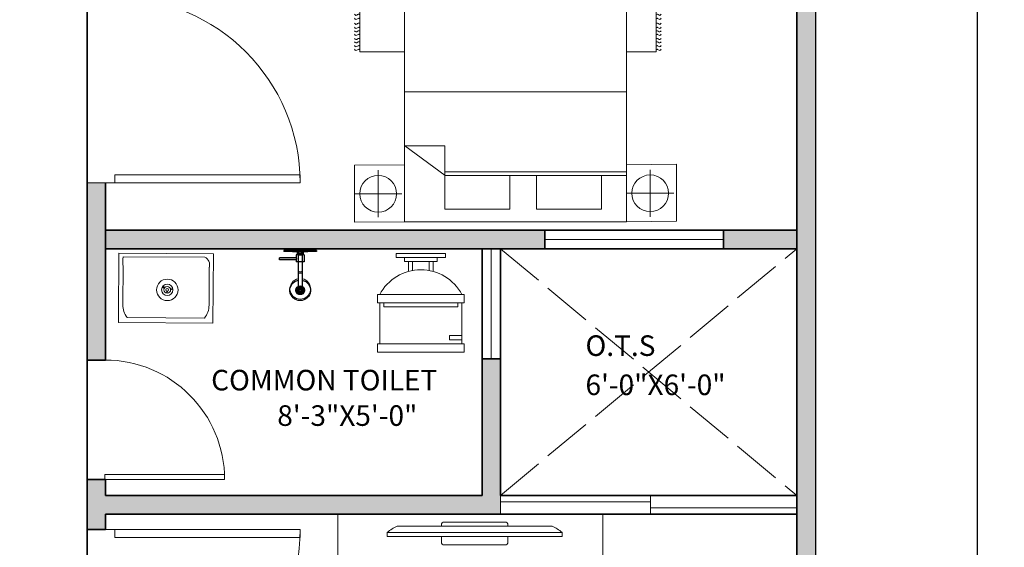
# Model space of a CAD drawing. Units: inches. Extents: x 0 to 4258, y 0 to 3769.
# Tile 26 of 30: x 3845 to 4085, y 3385 to 3513. Entities that reach past the tile are written whole.
import ezdxf

# ---------------------------------------------------------------- set-up
doc = ezdxf.new("R2010")
doc.units = ezdxf.units.IN
doc.header["$MEASUREMENT"] = 0
doc.linetypes.add('ACAD_ISO02W100', pattern=[15, 12, -3])
doc.layers.get('0').update_dxf_attribs({"color": 16})
for name, color, linetype, lineweight in [('A-ANNO-DIMS', 250, 'Continuous', 18), ('A-AREA-IDEN', 250, 'Continuous', 18), ('A-EQPM', 8, 'Continuous', 18), ('A-FLOR-FIXT', 250, 'Continuous', 18), ('A-FLOR-OVHD', 150, 'ACAD_ISO02W100', 13), ('A-WALL-PATT', 16, 'Continuous', 13), ('C-PROP', 150, 'Continuous', 25), ('doors', 250, 'Continuous', 18), ('furniture', 13, 'Continuous', 18), ('walls', 251, 'Continuous', 35), ('windows', 121, 'Continuous', 18)]:
    doc.layers.add(name, color=color, linetype=linetype, lineweight=lineweight)
doc.layers.add('PLUMBING FIXTURES', color=250, linetype='Continuous')
doc.styles.get("Standard").update_dxf_attribs({"font": 'arial.ttf'})
doc.dimstyles.get("Standard").update_dxf_attribs({"dimtxt": 7, "dimasz": 0.18, "dimexe": 0.18, "dimexo": 0.0625, "dimgap": 0.09, "dimtad": 0, "dimtih": 1, "dimtoh": 1, "dimzin": 0, "dimdsep": 46, "dimlunit": 3, "dimtxsty": 'Standard', "dimcen": 0.09, "dimadec": 0, "dimazin": 0, "dimtfac": 1, "dimtofl": 0, "dimtmove": 0, "dimatfit": 3, "dimfxl": 1, "dimtolj": 1, "dimtzin": 0, "dimarcsym": 0})

# ---------------------------------------------------------------- blocks, each defined once
blk = doc.blocks.new('CARPET')
at = {"layer": 'furniture'}
for p, q in [((-51.53, -98.11), (-51.53, -55.12)), ((-51.53, -55.12), (-41.27, -55.12)), ((36, -55.12), (51.55, -55.12)), ((51.55, -55.12), (51.55, -98.11)), ((51.55, -98.11), (-51.53, -98.11))]:
    blk.add_line(p, q, dxfattribs=at)
for points, knots in [([(-53.37, -55.99), (-53.22, -55.8), (-52.9, -55.41), (-52.34, -55.8), (-51.89, -56.08), (-51.65, -55.91), (-51.53, -55.83)], [0, 0, 0, 0, 0.653278, 1.290138, 1.740457, 2.114451, 2.114451, 2.114451, 2.114451]), ([(-53.37, -57.26), (-53.22, -57.07), (-52.9, -56.67), (-52.34, -57.07), (-51.89, -57.35), (-51.65, -57.17), (-51.53, -57.1)], [0, 0, 0, 0, 0.653278, 1.290138, 1.740457, 2.114451, 2.114451, 2.114451, 2.114451]), ([(-53.37, -58.59), (-53.22, -58.4), (-52.9, -58.01), (-52.34, -58.4), (-51.89, -58.68), (-51.65, -58.5), (-51.53, -58.43)], [0, 0, 0, 0, 0.653278, 1.290138, 1.740457, 2.114451, 2.114451, 2.114451, 2.114451]), ([(53.37, -55.99), (53.22, -55.8), (52.9, -55.41), (52.34, -55.8), (51.89, -56.08), (51.65, -55.91), (51.53, -55.83)], [0, 0, 0, 0, 0.653278, 1.290138, 1.740457, 2.114451, 2.114451, 2.114451, 2.114451]), ([(53.37, -57.26), (53.22, -57.07), (52.9, -56.67), (52.34, -57.07), (51.89, -57.35), (51.65, -57.17), (51.53, -57.1)], [0, 0, 0, 0, 0.653278, 1.290138, 1.740457, 2.114451, 2.114451, 2.114451, 2.114451]), ([(53.37, -58.59), (53.22, -58.4), (52.9, -58.01), (52.34, -58.4), (51.89, -58.68), (51.65, -58.5), (51.53, -58.43)], [0, 0, 0, 0, 0.653278, 1.290138, 1.740457, 2.114451, 2.114451, 2.114451, 2.114451]), ([(-53.37, -59.78), (-53.22, -59.58), (-52.9, -59.19), (-52.34, -59.58), (-51.89, -59.86), (-51.65, -59.69), (-51.53, -59.61)], [0, 0, 0, 0, 0.653278, 1.290138, 1.740457, 2.114451, 2.114451, 2.114451, 2.114451]), ([(-53.37, -61.22), (-53.22, -61.02), (-52.9, -60.63), (-52.34, -61.02), (-51.89, -61.3), (-51.65, -61.13), (-51.53, -61.05)], [0, 0, 0, 0, 0.653278, 1.290138, 1.740457, 2.114451, 2.114451, 2.114451, 2.114451]), ([(53.37, -59.78), (53.22, -59.58), (52.9, -59.19), (52.34, -59.58), (51.89, -59.86), (51.65, -59.69), (51.53, -59.61)], [0, 0, 0, 0, 0.653278, 1.290138, 1.740457, 2.114451, 2.114451, 2.114451, 2.114451]), ([(53.37, -61.22), (53.22, -61.02), (52.9, -60.63), (52.34, -61.02), (51.89, -61.3), (51.65, -61.13), (51.53, -61.05)], [0, 0, 0, 0, 0.653278, 1.290138, 1.740457, 2.114451, 2.114451, 2.114451, 2.114451]), ([(-53.37, -62.44), (-53.22, -62.25), (-52.9, -61.86), (-52.34, -62.25), (-51.89, -62.53), (-51.65, -62.36), (-51.53, -62.28)], [0, 0, 0, 0, 0.653278, 1.290138, 1.740457, 2.114451, 2.114451, 2.114451, 2.114451]), ([(-53.37, -63.63), (-53.22, -63.43), (-52.9, -63.04), (-52.34, -63.43), (-51.89, -63.72), (-51.65, -63.54), (-51.53, -63.46)], [0, 0, 0, 0, 0.653278, 1.290138, 1.740457, 2.114451, 2.114451, 2.114451, 2.114451]), ([(-53.37, -65.07), (-53.22, -64.87), (-52.9, -64.48), (-52.34, -64.87), (-51.89, -65.15), (-51.65, -64.98), (-51.53, -64.9)], [0, 0, 0, 0, 0.653278, 1.290138, 1.740457, 2.114451, 2.114451, 2.114451, 2.114451]), ([(53.37, -62.44), (53.22, -62.25), (52.9, -61.86), (52.34, -62.25), (51.89, -62.53), (51.65, -62.36), (51.53, -62.28)], [0, 0, 0, 0, 0.653278, 1.290138, 1.740457, 2.114451, 2.114451, 2.114451, 2.114451]), ([(53.37, -63.63), (53.22, -63.43), (52.9, -63.04), (52.34, -63.43), (51.89, -63.72), (51.65, -63.54), (51.53, -63.46)], [0, 0, 0, 0, 0.653278, 1.290138, 1.740457, 2.114451, 2.114451, 2.114451, 2.114451]), ([(53.37, -65.07), (53.22, -64.87), (52.9, -64.48), (52.34, -64.87), (51.89, -65.15), (51.65, -64.98), (51.53, -64.9)], [0, 0, 0, 0, 0.653278, 1.290138, 1.740457, 2.114451, 2.114451, 2.114451, 2.114451]), ([(-53.37, -66.76), (-53.22, -66.56), (-52.9, -66.17), (-52.34, -66.56), (-51.89, -66.84), (-51.65, -66.67), (-51.53, -66.59)], [0, 0, 0, 0, 0.653278, 1.290138, 1.740457, 2.114451, 2.114451, 2.114451, 2.114451]), ([(-53.37, -68.2), (-53.22, -68), (-52.9, -67.61), (-52.34, -68), (-51.89, -68.28), (-51.65, -68.11), (-51.53, -68.03)], [0, 0, 0, 0, 0.653278, 1.290138, 1.740457, 2.114451, 2.114451, 2.114451, 2.114451]), ([(53.37, -66.76), (53.22, -66.56), (52.9, -66.17), (52.34, -66.56), (51.89, -66.84), (51.65, -66.67), (51.53, -66.59)], [0, 0, 0, 0, 0.653278, 1.290138, 1.740457, 2.114451, 2.114451, 2.114451, 2.114451]), ([(53.37, -68.2), (53.22, -68), (52.9, -67.61), (52.34, -68), (51.89, -68.28), (51.65, -68.11), (51.53, -68.03)], [0, 0, 0, 0, 0.653278, 1.290138, 1.740457, 2.114451, 2.114451, 2.114451, 2.114451]), ([(-53.37, -69.53), (-53.22, -69.33), (-52.9, -68.94), (-52.34, -69.33), (-51.89, -69.61), (-51.65, -69.44), (-51.53, -69.36)], [0, 0, 0, 0, 0.653278, 1.290138, 1.740457, 2.114451, 2.114451, 2.114451, 2.114451]), ([(-53.37, -70.79), (-53.22, -70.6), (-52.9, -70.21), (-52.34, -70.6), (-51.89, -70.88), (-51.65, -70.7), (-51.53, -70.63)], [0, 0, 0, 0, 0.653278, 1.290138, 1.740457, 2.114451, 2.114451, 2.114451, 2.114451]), ([(-53.37, -72.12), (-53.22, -71.93), (-52.9, -71.54), (-52.34, -71.93), (-51.89, -72.21), (-51.65, -72.04), (-51.53, -71.96)], [0, 0, 0, 0, 0.653278, 1.290138, 1.740457, 2.114451, 2.114451, 2.114451, 2.114451]), ([(53.37, -69.53), (53.22, -69.33), (52.9, -68.94), (52.34, -69.33), (51.89, -69.61), (51.65, -69.44), (51.53, -69.36)], [0, 0, 0, 0, 0.653278, 1.290138, 1.740457, 2.114451, 2.114451, 2.114451, 2.114451]), ([(53.37, -70.79), (53.22, -70.6), (52.9, -70.21), (52.34, -70.6), (51.89, -70.88), (51.65, -70.7), (51.53, -70.63)], [0, 0, 0, 0, 0.653278, 1.290138, 1.740457, 2.114451, 2.114451, 2.114451, 2.114451]), ([(53.37, -72.12), (53.22, -71.93), (52.9, -71.54), (52.34, -71.93), (51.89, -72.21), (51.65, -72.04), (51.53, -71.96)], [0, 0, 0, 0, 0.653278, 1.290138, 1.740457, 2.114451, 2.114451, 2.114451, 2.114451]), ([(-53.37, -73.31), (-53.22, -73.11), (-52.9, -72.72), (-52.34, -73.11), (-51.89, -73.4), (-51.65, -73.22), (-51.53, -73.14)], [0, 0, 0, 0, 0.653278, 1.290138, 1.740457, 2.114451, 2.114451, 2.114451, 2.114451]), ([(-53.37, -74.75), (-53.22, -74.55), (-52.9, -74.16), (-52.34, -74.55), (-51.89, -74.83), (-51.65, -74.66), (-51.53, -74.58)], [0, 0, 0, 0, 0.653278, 1.290138, 1.740457, 2.114451, 2.114451, 2.114451, 2.114451]), ([(53.37, -73.31), (53.22, -73.11), (52.9, -72.72), (52.34, -73.11), (51.89, -73.4), (51.65, -73.22), (51.53, -73.14)], [0, 0, 0, 0, 0.653278, 1.290138, 1.740457, 2.114451, 2.114451, 2.114451, 2.114451]), ([(53.37, -74.75), (53.22, -74.55), (52.9, -74.16), (52.34, -74.55), (51.89, -74.83), (51.65, -74.66), (51.53, -74.58)], [0, 0, 0, 0, 0.653278, 1.290138, 1.740457, 2.114451, 2.114451, 2.114451, 2.114451]), ([(-53.37, -75.98), (-53.22, -75.78), (-52.9, -75.39), (-52.34, -75.78), (-51.89, -76.06), (-51.65, -75.89), (-51.53, -75.81)], [0, 0, 0, 0, 0.653278, 1.290138, 1.740457, 2.114451, 2.114451, 2.114451, 2.114451]), ([(-53.37, -77.16), (-53.22, -76.96), (-52.9, -76.57), (-52.34, -76.96), (-51.89, -77.25), (-51.65, -77.07), (-51.53, -76.99)], [0, 0, 0, 0, 0.653278, 1.290138, 1.740457, 2.114451, 2.114451, 2.114451, 2.114451]), ([(-53.37, -78.6), (-53.22, -78.4), (-52.9, -78.01), (-52.34, -78.4), (-51.89, -78.68), (-51.65, -78.51), (-51.53, -78.43)], [0, 0, 0, 0, 0.653278, 1.290138, 1.740457, 2.114451, 2.114451, 2.114451, 2.114451]), ([(53.37, -75.98), (53.22, -75.78), (52.9, -75.39), (52.34, -75.78), (51.89, -76.06), (51.65, -75.89), (51.53, -75.81)], [0, 0, 0, 0, 0.653278, 1.290138, 1.740457, 2.114451, 2.114451, 2.114451, 2.114451]), ([(53.37, -77.16), (53.22, -76.96), (52.9, -76.57), (52.34, -76.96), (51.89, -77.25), (51.65, -77.07), (51.53, -76.99)], [0, 0, 0, 0, 0.653278, 1.290138, 1.740457, 2.114451, 2.114451, 2.114451, 2.114451]), ([(53.37, -78.6), (53.22, -78.4), (52.9, -78.01), (52.34, -78.4), (51.89, -78.68), (51.65, -78.51), (51.53, -78.43)], [0, 0, 0, 0, 0.653278, 1.290138, 1.740457, 2.114451, 2.114451, 2.114451, 2.114451]), ([(-53.37, -80.29), (-53.22, -80.09), (-52.9, -79.7), (-52.34, -80.09), (-51.89, -80.37), (-51.65, -80.2), (-51.53, -80.12)], [0, 0, 0, 0, 0.653278, 1.290138, 1.740457, 2.114451, 2.114451, 2.114451, 2.114451]), ([(-53.37, -81.73), (-53.22, -81.53), (-52.9, -81.14), (-52.34, -81.53), (-51.89, -81.81), (-51.65, -81.64), (-51.53, -81.56)], [0, 0, 0, 0, 0.653278, 1.290138, 1.740457, 2.114451, 2.114451, 2.114451, 2.114451]), ([(53.37, -80.29), (53.22, -80.09), (52.9, -79.7), (52.34, -80.09), (51.89, -80.37), (51.65, -80.2), (51.53, -80.12)], [0, 0, 0, 0, 0.653278, 1.290138, 1.740457, 2.114451, 2.114451, 2.114451, 2.114451]), ([(53.37, -81.73), (53.22, -81.53), (52.9, -81.14), (52.34, -81.53), (51.89, -81.81), (51.65, -81.64), (51.53, -81.56)], [0, 0, 0, 0, 0.653278, 1.290138, 1.740457, 2.114451, 2.114451, 2.114451, 2.114451]), ([(-53.37, -83.06), (-53.22, -82.86), (-52.9, -82.47), (-52.34, -82.86), (-51.89, -83.14), (-51.65, -82.97), (-51.53, -82.89)], [0, 0, 0, 0, 0.653278, 1.290138, 1.740457, 2.114451, 2.114451, 2.114451, 2.114451]), ([(-53.37, -84.18), (-53.22, -83.99), (-52.9, -83.6), (-52.34, -83.99), (-51.89, -84.27), (-51.65, -84.09), (-51.53, -84.02)], [0, 0, 0, 0, 0.653278, 1.290138, 1.740457, 2.114451, 2.114451, 2.114451, 2.114451]), ([(-53.37, -85.51), (-53.22, -85.32), (-52.9, -84.93), (-52.34, -85.32), (-51.89, -85.6), (-51.65, -85.42), (-51.53, -85.35)], [0, 0, 0, 0, 0.653278, 1.290138, 1.740457, 2.114451, 2.114451, 2.114451, 2.114451]), ([(53.37, -83.06), (53.22, -82.86), (52.9, -82.47), (52.34, -82.86), (51.89, -83.14), (51.65, -82.97), (51.53, -82.89)], [0, 0, 0, 0, 0.653278, 1.290138, 1.740457, 2.114451, 2.114451, 2.114451, 2.114451]), ([(53.37, -84.18), (53.22, -83.99), (52.9, -83.6), (52.34, -83.99), (51.89, -84.27), (51.65, -84.09), (51.53, -84.02)], [0, 0, 0, 0, 0.653278, 1.290138, 1.740457, 2.114451, 2.114451, 2.114451, 2.114451]), ([(53.37, -85.51), (53.22, -85.32), (52.9, -84.93), (52.34, -85.32), (51.89, -85.6), (51.65, -85.42), (51.53, -85.35)], [0, 0, 0, 0, 0.653278, 1.290138, 1.740457, 2.114451, 2.114451, 2.114451, 2.114451]), ([(-53.37, -86.7), (-53.22, -86.5), (-52.9, -86.11), (-52.34, -86.5), (-51.89, -86.78), (-51.65, -86.61), (-51.53, -86.53)], [0, 0, 0, 0, 0.653278, 1.290138, 1.740457, 2.114451, 2.114451, 2.114451, 2.114451]), ([(-53.37, -88.14), (-53.22, -87.94), (-52.9, -87.55), (-52.34, -87.94), (-51.89, -88.22), (-51.65, -88.05), (-51.53, -87.97)], [0, 0, 0, 0, 0.653278, 1.290138, 1.740457, 2.114451, 2.114451, 2.114451, 2.114451]), ([(-53.37, -89.36), (-53.22, -89.17), (-52.9, -88.78), (-52.34, -89.17), (-51.89, -89.45), (-51.65, -89.28), (-51.53, -89.2)], [0, 0, 0, 0, 0.653278, 1.290138, 1.740457, 2.114451, 2.114451, 2.114451, 2.114451]), ([(53.37, -86.7), (53.22, -86.5), (52.9, -86.11), (52.34, -86.5), (51.89, -86.78), (51.65, -86.61), (51.53, -86.53)], [0, 0, 0, 0, 0.653278, 1.290138, 1.740457, 2.114451, 2.114451, 2.114451, 2.114451]), ([(53.37, -88.14), (53.22, -87.94), (52.9, -87.55), (52.34, -87.94), (51.89, -88.22), (51.65, -88.05), (51.53, -87.97)], [0, 0, 0, 0, 0.653278, 1.290138, 1.740457, 2.114451, 2.114451, 2.114451, 2.114451]), ([(53.37, -89.36), (53.22, -89.17), (52.9, -88.78), (52.34, -89.17), (51.89, -89.45), (51.65, -89.28), (51.53, -89.2)], [0, 0, 0, 0, 0.653278, 1.290138, 1.740457, 2.114451, 2.114451, 2.114451, 2.114451]), ([(-53.37, -90.55), (-53.22, -90.35), (-52.9, -89.96), (-52.34, -90.35), (-51.89, -90.64), (-51.65, -90.46), (-51.53, -90.38)], [0, 0, 0, 0, 0.653278, 1.290138, 1.740457, 2.114451, 2.114451, 2.114451, 2.114451]), ([(-53.37, -91.99), (-53.22, -91.79), (-52.9, -91.4), (-52.34, -91.79), (-51.89, -92.07), (-51.65, -91.9), (-51.53, -91.82)], [0, 0, 0, 0, 0.653278, 1.290138, 1.740457, 2.114451, 2.114451, 2.114451, 2.114451]), ([(-53.37, -92.69), (-53.22, -92.48), (-52.9, -92.08), (-52.35, -92.49), (-51.89, -92.77), (-51.65, -92.6), (-51.53, -92.52)], [0, 0, 0, 0, 0.663904, 1.307406, 1.757725, 2.131719, 2.131719, 2.131719, 2.131719]), ([(53.37, -90.55), (53.22, -90.35), (52.9, -89.96), (52.34, -90.35), (51.9, -90.63), (51.66, -90.47), (51.55, -90.4)], [0, 0, 0, 0, 0.653278, 1.290138, 1.740457, 2.0926, 2.0926, 2.0926, 2.0926]), ([(53.37, -91.99), (53.22, -91.79), (52.9, -91.4), (52.34, -91.79), (51.9, -92.07), (51.66, -91.91), (51.55, -91.83)], [0, 0, 0, 0, 0.653278, 1.290138, 1.740457, 2.0926, 2.0926, 2.0926, 2.0926]), ([(53.37, -92.69), (53.22, -92.49), (52.9, -92.09), (52.34, -92.49), (51.9, -92.77), (51.66, -92.61), (51.55, -92.53)], [0, 0, 0, 0, 0.656792, 1.295826, 1.746145, 2.098292, 2.098292, 2.098292, 2.098292]), ([(-53.37, -93.61), (-53.22, -93.42), (-52.9, -93.03), (-52.34, -93.42), (-51.89, -93.7), (-51.65, -93.52), (-51.53, -93.45)], [0, 0, 0, 0, 0.653278, 1.290138, 1.740457, 2.114451, 2.114451, 2.114451, 2.114451]), ([(-53.37, -94.55), (-53.22, -94.35), (-52.9, -93.96), (-52.34, -94.35), (-51.89, -94.63), (-51.65, -94.46), (-51.53, -94.38)], [0, 0, 0, 0, 0.653278, 1.290138, 1.740457, 2.114451, 2.114451, 2.114451, 2.114451]), ([(-53.37, -95.05), (-53.22, -94.85), (-52.9, -94.46), (-52.34, -94.85), (-51.89, -95.14), (-51.65, -94.96), (-51.53, -94.88)], [0, 0, 0, 0, 0.653278, 1.290138, 1.740457, 2.114451, 2.114451, 2.114451, 2.114451]), ([(-53.37, -95.73), (-53.22, -95.54), (-52.9, -95.15), (-52.34, -95.54), (-51.89, -95.82), (-51.65, -95.65), (-51.53, -95.57)], [0, 0, 0, 0, 0.653278, 1.290138, 1.740457, 2.114451, 2.114451, 2.114451, 2.114451]), ([(53.37, -95.78), (53.22, -95.58), (52.9, -95.19), (52.34, -95.58), (51.89, -95.86), (51.65, -95.69), (51.53, -95.61)], [0, 0, 0, 0, 0.653278, 1.290138, 1.740457, 2.114451, 2.114451, 2.114451, 2.114451]), ([(53.37, -93.66), (53.22, -93.46), (52.9, -93.07), (52.34, -93.46), (51.9, -93.74), (51.66, -93.58), (51.55, -93.5)], [0, 0, 0, 0, 0.653278, 1.290138, 1.740457, 2.0926, 2.0926, 2.0926, 2.0926]), ([(53.37, -94.59), (53.22, -94.4), (52.9, -94.01), (52.34, -94.4), (51.9, -94.68), (51.66, -94.51), (51.55, -94.44)], [0, 0, 0, 0, 0.653278, 1.290138, 1.740457, 2.0926, 2.0926, 2.0926, 2.0926]), ([(53.37, -95.1), (53.22, -94.9), (52.9, -94.51), (52.34, -94.9), (51.9, -95.18), (51.66, -95.02), (51.55, -94.94)], [0, 0, 0, 0, 0.653278, 1.290138, 1.740457, 2.0926, 2.0926, 2.0926, 2.0926]), ([(-53.37, -96.38), (-53.22, -96.18), (-52.9, -95.79), (-52.34, -96.18), (-51.89, -96.47), (-51.65, -96.29), (-51.53, -96.21)], [0, 0, 0, 0, 0.653278, 1.290138, 1.740457, 2.114451, 2.114451, 2.114451, 2.114451]), ([(-53.37, -97.17), (-53.22, -96.98), (-52.9, -96.59), (-52.34, -96.98), (-51.89, -97.26), (-51.65, -97.08), (-51.53, -97.01)], [0, 0, 0, 0, 0.653278, 1.290138, 1.740457, 2.114451, 2.114451, 2.114451, 2.114451]), ([(-53.37, -97.99), (-53.22, -97.79), (-52.9, -97.4), (-52.34, -97.79), (-51.89, -98.08), (-51.65, -97.9), (-51.53, -97.82)], [0, 0, 0, 0, 0.653278, 1.290138, 1.740457, 2.114451, 2.114451, 2.114451, 2.114451]), ([(53.37, -96.43), (53.22, -96.23), (52.9, -95.84), (52.34, -96.23), (51.89, -96.51), (51.65, -96.34), (51.53, -96.26)], [0, 0, 0, 0, 0.653278, 1.290138, 1.740457, 2.114451, 2.114451, 2.114451, 2.114451]), ([(53.37, -97.22), (53.22, -97.02), (52.9, -96.63), (52.34, -97.02), (51.89, -97.3), (51.65, -97.13), (51.53, -97.05)], [0, 0, 0, 0, 0.653278, 1.290138, 1.740457, 2.114451, 2.114451, 2.114451, 2.114451]), ([(53.37, -97.99), (53.22, -97.79), (52.9, -97.4), (52.34, -97.79), (51.89, -98.08), (51.65, -97.9), (51.53, -97.82)], [0, 0, 0, 0, 0.653278, 1.290138, 1.740457, 2.114451, 2.114451, 2.114451, 2.114451])]:
    blk.add_open_spline(points, degree=3, knots=knots, dxfattribs=at)
blk = doc.blocks.new('A$C58D270C6')
at = {"layer": 'furniture'}
for p, q in [((9.09, 124.13), (9.09, 108.87)), ((1.46, 116.5), (16.73, 116.5)), ((14.97, 94.84), (24.62, 107.92)), ((24.62, 94.93), (24.62, 107.92)), ((42.08, 108), (42.08, 36)), ((14.97, 94.93), (24.62, 94.93)), ((14.97, 94.84), (14.97, 36)), ((16.22, 94.93), (16.22, 36)), ((9.25, 36), (9.25, 20.74)), ((1.62, 28.37), (16.88, 28.37))]:
    blk.add_line(p, q, dxfattribs=at)
for points in [[(18.5, 108), (18.34, 124.13), (-0.16, 124.13), (0, 108)], [(0, 108), (77.91, 108), (77.91, 36), (0, 36)], [(4.09, 94.93), (14.97, 94.93), (14.97, 73.83), (4.09, 73.83)], [(4.09, 65.23), (14.97, 65.23), (14.97, 44.13), (4.09, 44.13)], [(18.65, 19.87), (18.5, 36), (0, 36), (0.16, 19.87)]]:
    blk.add_lwpolyline(points, close=True, dxfattribs=at)
for centre in [(9.09, 116.5), (9.25, 28.37)]:
    blk.add_circle(centre, 5.95, dxfattribs=at)
at = {"layer": 'furniture', "xscale": 0.9312884925094044, "yscale": 0.9312884925094044, "zscale": 0.9312884925094044, "rotation": 90}
blk.add_blockref('CARPET', (3.79, 74.47), dxfattribs=at)
blk = doc.blocks.new('PLASMA-LARGE')
at = {"layer": 'furniture'}
for p, q in [((-7.26, 0), (7.26, 0)), ((-18.61, -1), (18.61, -1)), ((-8, -1), (-8, -0.74)), ((8, -1), (8, -0.74)), ((-21, -2.5), (21, -2.5)), ((-21, -2.5), (-21, -3.5)), ((-21, -3.5), (21, -3.5)), ((-8, -3.5), (-8, -4.76)), ((8, -3.5), (8, -4.76)), ((21, -2.5), (21, -3.5)), ((-7.26, -5.5), (7.26, -5.5))]:
    blk.add_line(p, q, dxfattribs=at)
for centre, radius, start, end in [((-7.26, -0.74), 0.744, 90, 180), ((7.26, -0.74), 0.744, 0, 90), ((-13.97, -11.05), 11.07, 114.7602, 129.4175), ((13.97, -11.05), 11.07, 50.5825, 65.2398), ((-7.26, -4.76), 0.744, 180, 270), ((7.26, -4.76), 0.744, 270, 0)]:
    blk.add_arc(centre, radius, start, end, dxfattribs=at)
blk = doc.blocks.new('*U18')
for p, q in [((-10, 22), (-10, 12)), ((10, 12), (10, 22)), ((-10, 21), (-7, 21)), ((-7, 20), (-10, 20)), ((-7, 21), (-7, 20)), ((10.5, 12), (-10.5, 12)), ((-10.5, 10), (-10.5, 12)), ((9, 13), (-9, 13)), ((-9, 13), (-9, 12)), ((9, 12), (9, 13)), ((10.5, 12), (10.5, 10)), ((10.5, 10), (-10.5, 10)), ((-3, 4.4065), (-3, 2)), ((-2, 2), (-2, 4.1658)), ((2, 4.1658), (2, 2)), ((3, 2), (3, 4.4065)), ((4, 2), (-4, 2)), ((-4, 2), (-4, 1)), ((4, 1), (4, 2))]:
    blk.add_line(p, q)
for points in [[(10.5, 22), (10.5, 24), (-10.5, 24), (-10.5, 22)], [(6, 0), (6, 1), (-6, 1), (-6, 0)]]:
    blk.add_lwpolyline(points, close=True)
blk.add_arc((0, 15.3333), 11.3333, 208.0725, 331.9275)
blk = doc.blocks.new('*U23')
for p, q in [((0, 0), (0, -6)), ((40, 0), (40, -6))]:
    blk.add_line(p, q)
blk.add_lwpolyline([(0, 0), (0, 40), (1.75, 40), (1.75, 0)], close=True)
blk.add_arc((0, 0), 40, 0, 90)
blk = doc.blocks.new('*D26')
at = {"layer": 'A-ANNO-DIMS', "color": 0, "lineweight": -2, "transparency": 16777216}
for p, q in [((4077.41, 3656.79), (4078.27, 3656.79)), ((4078.09, 3656.61), (4078.09, 3329.69)), ((4078.09, 2995.47), (4078.09, 3322.39)), ((4077.41, 2995.29), (4078.27, 2995.29))]:
    blk.add_line(p, q, dxfattribs=at)
at = {"layer": 'A-ANNO-DIMS', "color": 0, "transparency": 16777216}
for points in [[(4078.06, 3656.61), (4078.12, 3656.61), (4078.09, 3656.79)], [(4078.06, 2995.47), (4078.12, 2995.47), (4078.09, 2995.29)]]:
    blk.add_solid(points, dxfattribs=at)
at = {"layer": 'Defpoints', "color": 0, "transparency": 16777216}
for p in [(4077.35, 3656.79), (4077.35, 2995.29), (4078.09, 2995.29)]:
    blk.add_point(p, dxfattribs=at)
at = {"layer": 'A-ANNO-DIMS', "color": 0, "transparency": 16777216, "insert": (4078.09, 3326.04), "char_height": 7, "attachment_point": 5}
blk.add_mtext("\\A1;55'", dxfattribs=at)
blk = doc.blocks.new('BASIN-RECTANGULAR')
for p, q in [((0.01, 1.29), (0.11, 17)), ((0.11, 17), (23.11, 16.85)), ((23.11, 16.85), (23, 0)), ((1.16, 16.16), (21.05, 16.03)), ((1.14, 13.79), (1.08, 4.5)), ((22.11, 13.65), (22.05, 4.36)), ((11.13, 8.4), (10.74, 8.87)), ((11.26, 8.61), (10.89, 9.05)), ((11.75, 7.78), (11.7, 7.3)), ((11.88, 7.27), (11.94, 7.76)), ((12.59, 8.3), (13.23, 8.41)), ((12.71, 8.08), (13.27, 8.19)), ((0, 0.15), (0.01, 1.29)), ((23, 0), (0, 0.15)), ((2.14, 1.35), (20.95, 1.23))]:
    blk.add_line(p, q)
for radius in [2.61, 1.39, 0.816, 0.338]:
    blk.add_circle((11.89, 8.09), radius)
for centre, radius, start, end in [((10.4, 14.91), 9.33, 172.3124, 186.9318), ((20.1, 14.18), 2.08, 345.2338, 62.9258), ((6.48, 4.56), 5.4, 180.6949, 216.4918), ((16.65, 4.5), 5.4, 322.7525, 358.5493)]:
    blk.add_arc(centre, radius, start, end)
blk = doc.blocks.new('O.H SHOWER-PL')
at = {"layer": 'PLUMBING FIXTURES'}
for points in [[(-1.84, 0), (-1.84, -0.25), (1.84, -0.25), (1.84, 0)], [(0.46, -8.72), (0.46, -9.67, -0.422337), (-0.46, -9.67), (-0.46, -8.72, 4.325472)]]:
    blk.add_hatch(color=256, dxfattribs=at).paths.add_polyline_path(points)
for p, q in [((-1.84, 0), (-1.84, -0.25)), ((1.84, 0), (-1.84, 0)), ((1.84, 0), (1.84, -0.25)), ((1.84, -0.25), (-1.84, -0.25)), ((-0.46, -0.25), (-0.46, -9.67)), ((0.46, -0.25), (0.46, -9.67))]:
    blk.add_line(p, q, dxfattribs=at)
for centre, radius, start, end in [((0, -4.48), 1.03, 243.53, 296.47), ((0, -9.67), 2.5, 100.61, 79.39), ((0, -9.67), 1.05, 116.0349, 63.9652), ((0, -9.22), 0.643, 224.2078, 315.7922)]:
    blk.add_arc(centre, radius, start, end, dxfattribs=at)
blk = doc.blocks.new('DIVERTER-PL')
at = {"layer": 'PLUMBING FIXTURES'}
for points in [[(4, 0), (-4, 0), (-4, -0.25), (4, -0.25)], [(0.38, -1.14), (0.38, -0.7), (-0.37, -0.7), (-0.37, -1.14)], [(1, -1.75, 0.30818), (1, -2.25), (5, -2.25), (5, -1.75)]]:
    blk.add_hatch(color=256, dxfattribs=at).paths.add_polyline_path(points)
for p, q in [((-4, 0), (-4, -0.25)), ((-4, 0), (4, 0)), ((4, 0), (4, -0.25)), ((-4, -0.25), (4, -0.25)), ((-4, -0.25), (4, -0.25)), ((-1, -1.05), (-0.37, -1.05)), ((-1, -1.05), (-1, -2.75)), ((-0.75, -0.25), (-0.75, -1.05)), ((-0.37, -0.7), (0.38, -0.7)), ((-0.37, -0.7), (-0.37, -1.14)), ((-0.37, -1.14), (0.38, -1.14)), ((-0.32, -0.7), (-0.32, -0.25)), ((0.32, -0.7), (0.32, -0.25)), ((0.38, -0.7), (0.38, -1.14)), ((0.38, -1.05), (1, -1.05)), ((0.75, -0.25), (0.75, -1.05)), ((1, -1.05), (1, -1.75)), ((1, -2.25), (1, -2.75)), ((-1, -2.75), (1, -2.75))]:
    blk.add_line(p, q, dxfattribs=at)
at = {"layer": 'PLUMBING FIXTURES', "ltscale": 12}
for p, q in [((1, -1.75), (5, -1.75)), ((1, -2.25), (5, -2.25)), ((5, -2.25), (5, -1.75))]:
    blk.add_line(p, q, dxfattribs=at)
at = {"layer": 'PLUMBING FIXTURES'}
blk.add_arc((1.37, -2), 0.444, 145.7435, 214.2565, dxfattribs=at)
blk = doc.blocks.new('A$C7F153053')
at = {"layer": 'PLUMBING FIXTURES', "xscale": -1, "rotation": 270}
for name in ['DIVERTER-PL', 'O.H SHOWER-PL']:
    blk.add_blockref(name, (12.17, 4), dxfattribs=at)
blk = doc.blocks.new('SHOWER-WALL-SET')
blk.add_hatch(color=256).paths.add_polyline_path([(5.46, 1.56), (5.46, 2.5, 0.422337), (4.54, 2.5), (4.54, 1.56, -4.325472)])
blk.add_hatch(color=256).paths.add_polyline_path([(5.46, 1.56), (5.46, 2.5, 0.422337), (4.54, 2.5), (4.54, 1.56, -4.325472)])
blk.add_hatch(color=256).paths.add_polyline_path([(5.46, 1.56), (5.46, 2.5, 0.422337), (4.54, 2.5), (4.54, 1.56, -4.325472)])
blk.add_hatch(color=256).paths.add_polyline_path([(5.46, 1.56), (5.46, 2.5, 0.422337), (4.54, 2.5), (4.54, 1.56, -4.325472)])
blk.add_hatch(color=256).paths.add_polyline_path([(5.46, 1.56), (5.46, 2.5, 0.422337), (4.54, 2.5), (4.54, 1.56, -4.325472)])
blk.add_hatch(color=256).paths.add_polyline_path([(5.46, 1.56), (5.46, 2.5, 0.422337), (4.54, 2.5), (4.54, 1.56, -4.325472)])
blk.add_hatch(color=256).paths.add_polyline_path([(5.46, 1.56), (5.46, 2.5, 0.422337), (4.54, 2.5), (4.54, 1.56, -4.325472)])
blk.add_hatch(color=256).paths.add_polyline_path([(5.46, 1.56), (5.46, 2.5, 0.422337), (4.54, 2.5), (4.54, 1.56, -4.325472)])
blk.add_hatch(color=256).paths.add_polyline_path([(5.46, 1.56), (5.46, 2.5, 0.422337), (4.54, 2.5), (4.54, 1.56, -4.325472)])
blk.add_hatch(color=256).paths.add_polyline_path([(5.46, 1.56), (5.46, 2.5, 0.422337), (4.54, 2.5), (4.54, 1.56, -4.325472)])
blk.add_hatch(color=256).paths.add_polyline_path([(5.46, 1.56), (5.46, 2.5, 0.422337), (4.54, 2.5), (4.54, 1.56, -4.325472)])
blk.add_hatch(color=256).paths.add_polyline_path([(5.46, 1.56), (5.46, 2.5, 0.422337), (4.54, 2.5), (4.54, 1.56, -4.325472)])
blk.add_hatch(color=256).paths.add_polyline_path([(5.46, 1.56), (5.46, 2.5, 0.422337), (4.54, 2.5), (4.54, 1.56, -4.325472)])
blk.add_hatch(color=256).paths.add_polyline_path([(5.46, 1.56), (5.46, 2.5, 0.422337), (4.54, 2.5), (4.54, 1.56, -4.325472)])
blk.add_hatch(color=256).paths.add_polyline_path([(5.46, 1.56), (5.46, 2.5, 0.422337), (4.54, 2.5), (4.54, 1.56, -4.325472)])
blk.add_hatch(color=256).paths.add_polyline_path([(5.46, 1.56), (5.46, 2.5, 0.422337), (4.54, 2.5), (4.54, 1.56, -4.325472)])
blk.add_hatch(color=256).paths.add_polyline_path([(5.46, 1.56), (5.46, 2.5, 0.422337), (4.54, 2.5), (4.54, 1.56, -4.325472)])
blk.add_hatch(color=256).paths.add_polyline_path([(5.46, 1.56), (5.46, 2.5, 0.422337), (4.54, 2.5), (4.54, 1.56, -4.325472)])
blk.add_hatch(color=256).paths.add_polyline_path([(5.46, 1.56), (5.46, 2.5, 0.422337), (4.54, 2.5), (4.54, 1.56, -4.325472)])
blk.add_hatch(color=256).paths.add_polyline_path([(5.46, 1.56), (5.46, 2.5, 0.422337), (4.54, 2.5), (4.54, 1.56, -4.325472)])
blk.add_hatch(color=256).paths.add_polyline_path([(5.46, 1.56), (5.46, 2.5, 0.422337), (4.54, 2.5), (4.54, 1.56, -4.325472)])
blk.add_hatch(color=256).paths.add_polyline_path([(5.46, 1.56), (5.46, 2.5, 0.422337), (4.54, 2.5), (4.54, 1.56, -4.325472)])
blk.add_hatch(color=256).paths.add_polyline_path([(5.46, 1.56), (5.46, 2.5, 0.422337), (4.54, 2.5), (4.54, 1.56, -4.325472)])
blk.add_hatch(color=256).paths.add_polyline_path([(5.46, 1.56), (5.46, 2.5, 0.422337), (4.54, 2.5), (4.54, 1.56, -4.325472)])
blk.add_hatch(color=256).paths.add_polyline_path([(5.46, 1.56), (5.46, 2.5, 0.422337), (4.54, 2.5), (4.54, 1.56, -4.325472)])
blk.add_hatch(color=256).paths.add_polyline_path([(5.46, 1.56), (5.46, 2.5, 0.422337), (4.54, 2.5), (4.54, 1.56, -4.325472)])
blk.add_hatch(color=256).paths.add_polyline_path([(5.46, 1.56), (5.46, 2.5, 0.422337), (4.54, 2.5), (4.54, 1.56, -4.325472)])
blk.add_hatch(color=256).paths.add_polyline_path([(5.46, 1.56), (5.46, 2.5, 0.422337), (4.54, 2.5), (4.54, 1.56, -4.325472)])
blk.add_hatch(color=256).paths.add_polyline_path([(5.46, 1.56), (5.46, 2.5, 0.422337), (4.54, 2.5), (4.54, 1.56, -4.325472)])
blk.add_hatch(color=256).paths.add_polyline_path([(5.46, 1.56), (5.46, 2.5, 0.422337), (4.54, 2.5), (4.54, 1.56, -4.325472)])
blk.add_hatch(color=256).paths.add_polyline_path([(5.46, 1.56), (5.46, 2.5, 0.422337), (4.54, 2.5), (4.54, 1.56, -4.325472)])
blk.add_hatch(color=256).paths.add_polyline_path([(5.46, 1.56), (5.46, 2.5, 0.422337), (4.54, 2.5), (4.54, 1.56, -4.325472)])
blk.add_hatch(color=256).paths.add_polyline_path([(5.46, 1.56), (5.46, 2.5, 0.422337), (4.54, 2.5), (4.54, 1.56, -4.325472)])
blk.add_hatch(color=256).paths.add_polyline_path([(5.46, 1.56), (5.46, 2.5, 0.422337), (4.54, 2.5), (4.54, 1.56, -4.325472)])
blk.add_hatch(color=256).paths.add_polyline_path([(5.46, 1.56), (5.46, 2.5, 0.422337), (4.54, 2.5), (4.54, 1.56, -4.325472)])
blk.add_hatch(color=256).paths.add_polyline_path([(5.46, 1.56), (5.46, 2.5, 0.422337), (4.54, 2.5), (4.54, 1.56, -4.325472)])
blk.add_hatch(color=256).paths.add_polyline_path([(5.46, 1.56), (5.46, 2.5, 0.422337), (4.54, 2.5), (4.54, 1.56, -4.325472)])
blk.add_hatch(color=256).paths.add_polyline_path([(5.46, 1.56), (5.46, 2.5, 0.422337), (4.54, 2.5), (4.54, 1.56, -4.325472)])
for p, q in [((4.54, 11.92), (4.54, 2.5)), ((4.54, 11.92), (4.54, 2.5)), ((4.54, 11.92), (4.54, 2.5)), ((4.54, 11.92), (4.54, 2.5)), ((4.54, 11.92), (4.54, 2.5)), ((4.54, 11.92), (4.54, 2.5)), ((4.54, 11.92), (4.54, 2.5)), ((4.54, 11.92), (4.54, 2.5)), ((4.54, 11.92), (4.54, 2.5)), ((4.54, 11.92), (4.54, 2.5)), ((4.54, 11.92), (4.54, 2.5)), ((4.54, 11.92), (4.54, 2.5)), ((4.54, 11.92), (4.54, 2.5)), ((4.54, 11.92), (4.54, 2.5)), ((4.54, 11.92), (4.54, 2.5)), ((4.54, 11.92), (4.54, 2.5)), ((4.54, 11.92), (4.54, 2.5)), ((4.54, 11.92), (4.54, 2.5)), ((4.54, 11.92), (4.54, 2.5)), ((4.54, 11.92), (4.54, 2.5)), ((4.54, 11.92), (4.54, 2.5)), ((4.54, 11.92), (4.54, 2.5)), ((4.54, 11.92), (4.54, 2.5)), ((4.54, 11.92), (4.54, 2.5)), ((4.54, 11.92), (4.54, 2.5)), ((4.54, 11.92), (4.54, 2.5)), ((4.54, 11.92), (4.54, 2.5)), ((4.54, 11.92), (4.54, 2.5)), ((4.54, 11.92), (4.54, 2.5)), ((4.54, 11.92), (4.54, 2.5)), ((4.54, 11.92), (4.54, 2.5)), ((4.54, 11.92), (4.54, 2.5)), ((4.54, 11.92), (4.54, 2.5)), ((4.54, 11.92), (4.54, 2.5)), ((4.54, 11.92), (4.54, 2.5)), ((4.54, 11.92), (4.54, 2.5)), ((4.54, 11.92), (4.54, 2.5)), ((4.54, 11.92), (4.54, 2.5)), ((5.46, 11.92), (5.46, 2.5)), ((5.46, 11.92), (5.46, 2.5)), ((5.46, 11.92), (5.46, 2.5)), ((5.46, 11.92), (5.46, 2.5)), ((5.46, 11.92), (5.46, 2.5)), ((5.46, 11.92), (5.46, 2.5)), ((5.46, 11.92), (5.46, 2.5)), ((5.46, 11.92), (5.46, 2.5)), ((5.46, 11.92), (5.46, 2.5)), ((5.46, 11.92), (5.46, 2.5)), ((5.46, 11.92), (5.46, 2.5)), ((5.46, 11.92), (5.46, 2.5)), ((5.46, 11.92), (5.46, 2.5)), ((5.46, 11.92), (5.46, 2.5)), ((5.46, 11.92), (5.46, 2.5)), ((5.46, 11.92), (5.46, 2.5)), ((5.46, 11.92), (5.46, 2.5)), ((5.46, 11.92), (5.46, 2.5)), ((5.46, 11.92), (5.46, 2.5)), ((5.46, 11.92), (5.46, 2.5)), ((5.46, 11.92), (5.46, 2.5)), ((5.46, 11.92), (5.46, 2.5)), ((5.46, 11.92), (5.46, 2.5)), ((5.46, 11.92), (5.46, 2.5)), ((5.46, 11.92), (5.46, 2.5)), ((5.46, 11.92), (5.46, 2.5)), ((5.46, 11.92), (5.46, 2.5)), ((5.46, 11.92), (5.46, 2.5)), ((5.46, 11.92), (5.46, 2.5)), ((5.46, 11.92), (5.46, 2.5)), ((5.46, 11.92), (5.46, 2.5)), ((5.46, 11.92), (5.46, 2.5)), ((5.46, 11.92), (5.46, 2.5)), ((5.46, 11.92), (5.46, 2.5)), ((5.46, 11.92), (5.46, 2.5)), ((5.46, 11.92), (5.46, 2.5)), ((5.46, 11.92), (5.46, 2.5)), ((5.46, 11.92), (5.46, 2.5))]:
    blk.add_line(p, q)
for centre, radius, start, end in [((5.01, 2.85), 2.5, 100.61, 79.39), ((5.01, 2.85), 2.5, 100.61, 79.39), ((5.01, 2.85), 2.5, 100.61, 79.39), ((5.01, 2.85), 2.5, 100.61, 79.39), ((5.01, 2.85), 2.5, 100.61, 79.39), ((5.01, 2.85), 2.5, 100.61, 79.39), ((5.01, 2.85), 2.5, 100.61, 79.39), ((5.01, 2.85), 2.5, 100.61, 79.39), ((5.01, 2.85), 2.5, 100.61, 79.39), ((5.01, 2.85), 2.5, 100.61, 79.39), ((5.01, 2.85), 2.5, 100.61, 79.39), ((5.01, 2.85), 2.5, 100.61, 79.39), ((5.01, 2.85), 2.5, 100.61, 79.39), ((5.01, 2.85), 2.5, 100.61, 79.39), ((5.01, 2.85), 2.5, 100.61, 79.39), ((5.01, 2.85), 2.5, 100.61, 79.39), ((5.01, 2.85), 2.5, 100.61, 79.39), ((5.01, 2.85), 2.5, 100.61, 79.39), ((5.01, 2.85), 2.5, 100.61, 79.39), ((5.01, 2.85), 2.5, 100.61, 79.39), ((5.01, 2.85), 2.5, 100.61, 79.39), ((5.01, 2.85), 2.5, 100.61, 79.39), ((5.01, 2.85), 2.5, 100.61, 79.39), ((5.01, 2.85), 2.5, 100.61, 79.39), ((5.01, 2.85), 2.5, 100.61, 79.39), ((5.01, 2.85), 2.5, 100.61, 79.39), ((5.01, 2.85), 2.5, 100.61, 79.39), ((5.01, 2.85), 2.5, 100.61, 79.39), ((5.01, 2.85), 2.5, 100.61, 79.39), ((5.01, 2.85), 2.5, 100.61, 79.39), ((5.01, 2.85), 2.5, 100.61, 79.39), ((5.01, 2.85), 2.5, 100.61, 79.39), ((5.01, 2.85), 2.5, 100.61, 79.39), ((5.01, 2.85), 2.5, 100.61, 79.39), ((5.01, 2.85), 2.5, 100.61, 79.39), ((5.01, 2.85), 2.5, 100.61, 79.39), ((5.01, 2.85), 2.5, 100.61, 79.39), ((5.01, 2.85), 2.5, 100.61, 79.39), ((5.01, 8.04), 1.03, 243.53, 296.47), ((5.01, 8.04), 1.03, 243.53, 296.47), ((5.01, 8.04), 1.03, 243.53, 296.47), ((5.01, 8.04), 1.03, 243.53, 296.47), ((5.01, 8.04), 1.03, 243.53, 296.47), ((5.01, 8.04), 1.03, 243.53, 296.47), ((5.01, 8.04), 1.03, 243.53, 296.47), ((5.01, 8.04), 1.03, 243.53, 296.47), ((5.01, 8.04), 1.03, 243.53, 296.47), ((5.01, 8.04), 1.03, 243.53, 296.47), ((5.01, 8.04), 1.03, 243.53, 296.47), ((5.01, 8.04), 1.03, 243.53, 296.47), ((5.01, 8.04), 1.03, 243.53, 296.47), ((5.01, 8.04), 1.03, 243.53, 296.47), ((5.01, 8.04), 1.03, 243.53, 296.47), ((5.01, 8.04), 1.03, 243.53, 296.47), ((5.01, 8.04), 1.03, 243.53, 296.47), ((5.01, 8.04), 1.03, 243.53, 296.47), ((5.01, 8.04), 1.03, 243.53, 296.47), ((5.01, 8.04), 1.03, 243.53, 296.47), ((5.01, 8.04), 1.03, 243.53, 296.47), ((5.01, 8.04), 1.03, 243.53, 296.47), ((5.01, 8.04), 1.03, 243.53, 296.47), ((5.01, 8.04), 1.03, 243.53, 296.47), ((5.01, 8.04), 1.03, 243.53, 296.47), ((5.01, 8.04), 1.03, 243.53, 296.47), ((5.01, 8.04), 1.03, 243.53, 296.47), ((5.01, 8.04), 1.03, 243.53, 296.47), ((5.01, 8.04), 1.03, 243.53, 296.47), ((5.01, 8.04), 1.03, 243.53, 296.47), ((5.01, 8.04), 1.03, 243.53, 296.47), ((5.01, 8.04), 1.03, 243.53, 296.47), ((5.01, 8.04), 1.03, 243.53, 296.47), ((5.01, 8.04), 1.03, 243.53, 296.47), ((5.01, 8.04), 1.03, 243.53, 296.47), ((5.01, 8.04), 1.03, 243.53, 296.47), ((5.01, 8.04), 1.03, 243.53, 296.47), ((5.01, 8.04), 1.03, 243.53, 296.47), ((5, 2.5), 1.05, 296.0348, 243.9651), ((5, 2.5), 1.05, 296.0348, 243.9651), ((5, 2.5), 1.05, 296.0348, 243.9651), ((5, 2.5), 1.05, 296.0348, 243.9651), ((5, 2.5), 1.05, 296.0348, 243.9651), ((5, 2.5), 1.05, 296.0348, 243.9651), ((5, 2.5), 1.05, 296.0348, 243.9651), ((5, 2.5), 1.05, 296.0348, 243.9651), ((5, 2.5), 1.05, 296.0348, 243.9651), ((5, 2.5), 1.05, 296.0348, 243.9651), ((5, 2.5), 1.05, 296.0348, 243.9651), ((5, 2.5), 1.05, 296.0348, 243.9651), ((5, 2.5), 1.05, 296.0348, 243.9651), ((5, 2.5), 1.05, 296.0348, 243.9651), ((5, 2.5), 1.05, 296.0348, 243.9651), ((5, 2.5), 1.05, 296.0348, 243.9651), ((5, 2.5), 1.05, 296.0348, 243.9651), ((5, 2.5), 1.05, 296.0348, 243.9651), ((5, 2.5), 1.05, 296.0348, 243.9651), ((5, 2.5), 1.05, 296.0348, 243.9651), ((5, 2.5), 1.05, 296.0348, 243.9651), ((5, 2.5), 1.05, 296.0348, 243.9651), ((5, 2.5), 1.05, 296.0348, 243.9651), ((5, 2.5), 1.05, 296.0348, 243.9651), ((5, 2.5), 1.05, 296.0348, 243.9651), ((5, 2.5), 1.05, 296.0348, 243.9651), ((5, 2.5), 1.05, 296.0348, 243.9651), ((5, 2.5), 1.05, 296.0348, 243.9651), ((5, 2.5), 1.05, 296.0348, 243.9651), ((5, 2.5), 1.05, 296.0348, 243.9651), ((5, 2.5), 1.05, 296.0348, 243.9651), ((5, 2.5), 1.05, 296.0348, 243.9651), ((5, 2.5), 1.05, 296.0348, 243.9651), ((5, 2.5), 1.05, 296.0348, 243.9651), ((5, 2.5), 1.05, 296.0348, 243.9651), ((5, 2.5), 1.05, 296.0348, 243.9651), ((5, 2.5), 1.05, 296.0348, 243.9651), ((5, 2.5), 1.05, 296.0348, 243.9651), ((5, 2.05), 0.643, 44.2078, 135.7922), ((5, 2.05), 0.643, 44.2078, 135.7922), ((5, 2.05), 0.643, 44.2078, 135.7922), ((5, 2.05), 0.643, 44.2078, 135.7922), ((5, 2.05), 0.643, 44.2078, 135.7922), ((5, 2.05), 0.643, 44.2078, 135.7922), ((5, 2.05), 0.643, 44.2078, 135.7922), ((5, 2.05), 0.643, 44.2078, 135.7922), ((5, 2.05), 0.643, 44.2078, 135.7922), ((5, 2.05), 0.643, 44.2078, 135.7922), ((5, 2.05), 0.643, 44.2078, 135.7922), ((5, 2.05), 0.643, 44.2078, 135.7922), ((5, 2.05), 0.643, 44.2078, 135.7922), ((5, 2.05), 0.643, 44.2078, 135.7922), ((5, 2.05), 0.643, 44.2078, 135.7922), ((5, 2.05), 0.643, 44.2078, 135.7922), ((5, 2.05), 0.643, 44.2078, 135.7922), ((5, 2.05), 0.643, 44.2078, 135.7922), ((5, 2.05), 0.643, 44.2078, 135.7922), ((5, 2.05), 0.643, 44.2078, 135.7922), ((5, 2.05), 0.643, 44.2078, 135.7922), ((5, 2.05), 0.643, 44.2078, 135.7922), ((5, 2.05), 0.643, 44.2078, 135.7922), ((5, 2.05), 0.643, 44.2078, 135.7922), ((5, 2.05), 0.643, 44.2078, 135.7922), ((5, 2.05), 0.643, 44.2078, 135.7922), ((5, 2.05), 0.643, 44.2078, 135.7922), ((5, 2.05), 0.643, 44.2078, 135.7922), ((5, 2.05), 0.643, 44.2078, 135.7922), ((5, 2.05), 0.643, 44.2078, 135.7922), ((5, 2.05), 0.643, 44.2078, 135.7922), ((5, 2.05), 0.643, 44.2078, 135.7922), ((5, 2.05), 0.643, 44.2078, 135.7922), ((5, 2.05), 0.643, 44.2078, 135.7922), ((5, 2.05), 0.643, 44.2078, 135.7922), ((5, 2.05), 0.643, 44.2078, 135.7922), ((5, 2.05), 0.643, 44.2078, 135.7922), ((5, 2.05), 0.643, 44.2078, 135.7922)]:
    blk.add_arc(centre, radius, start, end)
at = {"ltscale": 35, "rotation": 89.99999999999999}
blk.add_blockref('A$C7F153053', (9, 0), dxfattribs=at)
blk = doc.blocks.new('TV-CONSOLE-CABINET')
for p, q in [((0, 0), (0, 64.44)), ((0, 64.44), (14.9, 64.44)), ((14.9, 0), (0, 0))]:
    blk.add_line(p, q)

msp = doc.modelspace()

# ---------------------------------------------------------------- hatches: boundary and pattern name
at = {"layer": 'A-WALL-PATT'}
h = msp.add_hatch(color=256, dxfattribs=at)
h.dxf.hatch_style = 1
h.paths.add_polyline_path([(3866.304, 3343.984), (3861.804, 3343.984), (3861.804, 3251.848), (3866.304, 3251.848)])
h.paths.add_polyline_path([(3881.946, 3330.642), (3866.304, 3330.642), (3866.304, 3326.142), (3881.946, 3326.142)])
h.paths.add_polyline_path([(4038.804, 3656.793), (3933.804, 3656.793), (3933.804, 3638.769), (3938.304, 3638.769), (3938.304, 3652.293), (4034.304, 3652.293), (4034.304, 3260.793), (4030.207, 3260.793), (4030.207, 3256.293), (4038.804, 3256.293)])
h = msp.add_hatch(color=256, dxfattribs=at)
h.dxf.hatch_style = 1
h.paths.add_polyline_path([(3866.304, 3473.274), (3861.804, 3473.274), (3861.804, 3430.23), (3866.167, 3430.23, -0.001175), (3866.304, 3430.23)])
h = msp.add_hatch(color=256, dxfattribs=at)
h.dxf.hatch_style = 1
h.paths.add_polyline_path([(3687.804, 3163.293), (3678.804, 3163.293), (3678.804, 2995.293), (3687.804, 2995.293)])
h.paths.add_polyline_path([(3973.039, 3461.793), (3866.304, 3461.793), (3866.304, 3457.293), (3973.039, 3457.293)])
h.paths.add_polyline_path([(4034.304, 3461.793), (4016.474, 3461.793), (4016.474, 3457.293), (4034.304, 3457.293)])
h = msp.add_hatch(color=256, dxfattribs=at)
h.dxf.hatch_style = 1
h.paths.add_polyline_path([(3962.304, 3430.495), (3957.804, 3430.495), (3957.804, 3397.293), (3866.304, 3397.293), (3866.304, 3401.142), (3866.167, 3401.142), (3861.804, 3401.142), (3861.804, 3389.024), (3866.304, 3389.024), (3866.304, 3392.793), (3962.304, 3392.793), (3962.304, 3397.293)])

# ---------------------------------------------------------------- linework, layer by layer
at = {"layer": 'A-FLOR-OVHD'}
for p, q in [((3962.304, 3457.293), (4034.304, 3397.293)), ((3962.304, 3397.293), (4034.304, 3457.293))]:
    msp.add_line(p, q, dxfattribs=at)
at = {"layer": 'C-PROP'}
msp.add_line((4038.804, 3656.793), (4038.804, 2936.793), dxfattribs=at)
at = {"layer": 'walls'}
for p, q in [((4034.304, 3652.293), (4034.304, 3260.793)), ((3861.804, 3598.293), (3861.804, 3163.293)), ((3866.304, 3473.274), (3866.304, 3430.23)), ((3866.304, 3461.793), (4034.304, 3461.793)), ((3973.039, 3461.793), (3973.039, 3457.293)), ((4016.474, 3461.793), (4016.474, 3457.293)), ((3866.304, 3457.293), (4034.304, 3457.293)), ((3957.804, 3457.293), (3957.804, 3397.293)), ((3962.304, 3457.293), (3962.304, 3397.293)), ((3866.304, 3430.23), (3861.804, 3430.23)), ((3957.804, 3430.495), (3962.304, 3430.495)), ((3861.804, 3401.142), (3866.304, 3401.142)), ((3866.304, 3401.142), (3866.304, 3397.293)), ((3866.304, 3397.293), (3957.804, 3397.293)), ((3962.304, 3397.293), (4034.304, 3397.293)), ((3866.304, 3392.793), (4034.304, 3392.793)), ((3866.304, 3392.793), (3866.304, 3389.024)), ((3866.304, 3389.024), (3861.804, 3389.024))]:
    msp.add_line(p, q, dxfattribs=at)
at = {"layer": 'windows'}
for p, q in [((3973.039, 3461.793), (4016.474, 3461.793)), ((3973.039, 3459.543), (4016.474, 3459.543)), ((3957.804, 3430.495), (3957.804, 3457.293)), ((3960.054, 3430.495), (3960.054, 3457.293)), ((3962.304, 3430.495), (3962.304, 3457.293)), ((3973.039, 3457.293), (4016.474, 3457.293)), ((3962.304, 3397.293), (3962.304, 3392.793)), ((3962.304, 3395.785), (3998.753, 3395.785)), ((3998.753, 3392.793), (3998.753, 3397.293)), ((3998.753, 3394.313), (4034.304, 3394.313)), ((3962.304, 3392.793), (3998.753, 3392.793))]:
    msp.add_line(p, q, dxfattribs=at)

# ---------------------------------------------------------------- block references
at = {"layer": 'A-EQPM', "xscale": 1.011294184530666, "yscale": 1.011294184530666, "zscale": 1.011294184530666}
msp.add_blockref('PLASMA-LARGE', (3956.01, 3390.843), dxfattribs=at)
at = {"layer": 'A-FLOR-FIXT'}
for name, p in [('BASIN-RECTANGULAR', (3869.419, 3439.187)), ('SHOWER-WALL-SET', (3908.611, 3444.67))]:
    msp.add_blockref(name, p, dxfattribs=at)
at = {"layer": 'A-FLOR-FIXT', "rotation": 180}
msp.add_blockref('*U18', (3942.923, 3456.158), dxfattribs=at)
at = {"layer": 'doors', "rotation": 270}
for p, xscale, yscale, zscale in [((3868.56, 3473.274), -1.125993190768673, 1.125993190768673, 1.125993190768673), ((3866.167, 3401.142), -0.7272131312874193, 0.7272131312874193, 0.7272131312874193), ((3868.56, 3389.024), 1.125993190768673, 1.125993190768673, 1.125993190768673)]:
    msp.add_blockref('*U23', p, dxfattribs=dict(at, xscale=xscale, yscale=yscale, zscale=zscale))
at = {"layer": 'furniture', "xscale": 0.7500000390647866, "yscale": 0.7500000390647866, "zscale": 0.7500000390647866, "rotation": 90}
msp.add_blockref('A$C58D270C6', (4019.941, 3463.822), dxfattribs=at)
at = {"layer": 'furniture', "rotation": 89.99999999999704}
msp.add_blockref('TV-CONSOLE-CABINET', (3987.192, 3377.897), dxfattribs=at)

# ---------------------------------------------------------------- texts
at = {"layer": 'A-AREA-IDEN'}
for s, p in [('O.T.S', (3982.938, 3431.218)), (' COMMON TOILET', (3890.443, 3422.839)), ('6\'-0"X6\'-0"', (3982.938, 3421.703)), ('8\'-3"X5\'-0"', (3908.038, 3414.22))]:
    msp.add_text(s, height=5, dxfattribs=at).set_placement(p)

# ---------------------------------------------------------------- dimensions: what is measured, and where the dimension line sits
at = {"layer": 'A-ANNO-DIMS'}
dim = msp.add_linear_dim(base=(4078.091, 2995.293), p1=(4077.346, 3656.793), p2=(4077.346, 2995.293), angle=90, text="55'", dimstyle='Standard', override={"dimclrd": 0, "dimclre": 0, "dimclrt": 0}, dxfattribs=at)
dim.commit()
dim.dimension.update_dxf_attribs({"geometry": '*D26', "text_midpoint": (4078.091, 3326.043)})

doc.saveas('drawing.dxf')
